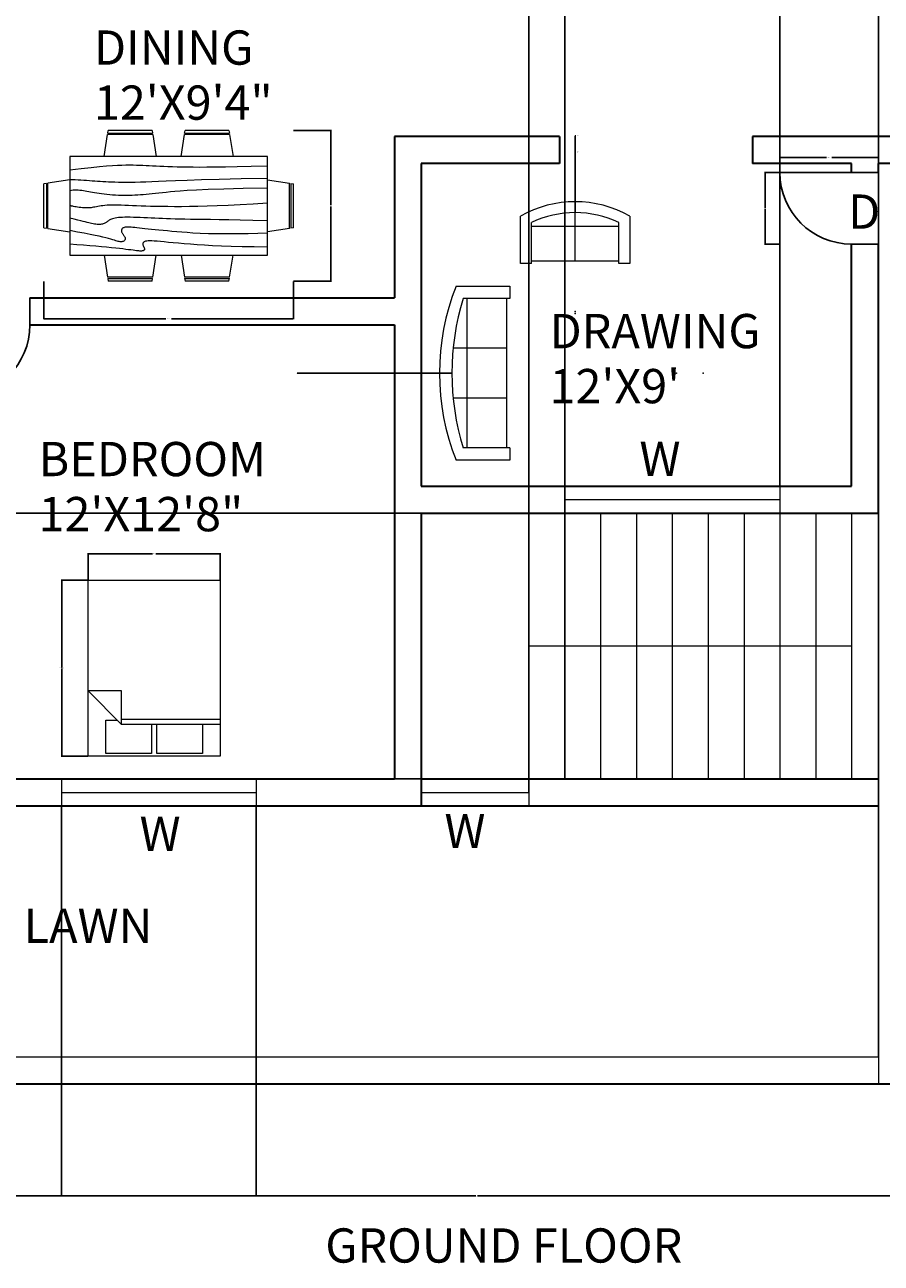
# Model space of a CAD drawing. Units: feet. Extents: x 1889 to 2708, y 1752 to 2375.
# Tile 2 of 5: x 2147 to 2434, y 1752 to 2166. Entities that reach past the tile are written whole.
import ezdxf

# ---------------------------------------------------------------- set-up
doc = ezdxf.new("R2010")
doc.units = ezdxf.units.FT
for name, color, linetype, lineweight in [('A-ANNO-DIMS', 2, 'Continuous', 18), ('A-ANNO-TEXT', 7, 'Continuous', 18), ('A-AREA-IDEN', 7, 'Continuous', 18), ('A-DOOR', 3, 'Continuous', 25), ('A-FLOR-STRS', 7, 'Continuous', 18), ('A-FURN', 8, 'Continuous', 18), ('A-GLAZ', 4, 'Continuous', 18), ('A-WALL', 7, 'Continuous', 35), ('C-PROP', 7, 'Continuous', 30), ('C-SITE', 94, 'Continuous', 18)]:
    doc.layers.add(name, color=color, linetype=linetype, lineweight=lineweight)
doc.styles.get("Standard").update_dxf_attribs({"font": 'arial.ttf'})
doc.dimstyles.get("Standard").update_dxf_attribs({"dimtxt": 0.18, "dimasz": 0.18, "dimexe": 0.18, "dimexo": 0.0625, "dimgap": 0.09, "dimtad": 0, "dimtih": 1, "dimtoh": 1, "dimdec": 4, "dimzin": 0, "dimdsep": 46, "dimtxsty": 'Standard', "dimcen": 0.09, "dimadec": 0, "dimazin": 0, "dimtfac": 1, "dimtdec": 4, "dimtofl": 0, "dimtmove": 0, "dimatfit": 3, "dimfxl": 1, "dimtolj": 1, "dimtzin": 0, "dimarcsym": 0})

# ---------------------------------------------------------------- blocks, each defined once
blk = doc.blocks.new('Dining Set - 36 x 72 in.')
for p, q in [((-22, 27.5), (-22.1562, 26.50042)), ((-22, 27.5), (-6, 27.5)), ((-5.8437, 26.49966), (-6, 27.5)), ((6, 27.5), (5.8438, 26.50042)), ((6, 27.5), (22, 27.5)), ((22.1563, 26.49966), (22, 27.5)), ((-22.2343, 26.00059), (-23.4847, 17.99762)), ((-22.2304, 26), (-5.7608, 26)), ((-5.8416, 26.5), (-22.1534, 26.5)), ((-4.5152, 17.99762), (-5.7655, 25.99926)), ((5.7657, 26.00059), (4.5153, 17.99762)), ((5.7696, 26), (22.2392, 26)), ((22.1584, 26.5), (5.8466, 26.5)), ((23.4848, 17.99762), (22.2345, 25.99926)), ((36, 18), (-36, 18)), ((-36, 18), (-36, -18)), ((36, -18), (36, 18)), ((-44.0006, 8.23428), (-35.9976, 9.48474)), ((44.0006, 8.23428), (35.9976, 9.48474)), ((-45.5, 8), (-44.5004, 8.15617)), ((-45.5, 8), (-45.5, -8)), ((-44.5, -8.15843), (-44.5, 8.15338)), ((-44, 8.23041), (-44, -8.23915)), ((44, 8.23041), (44, -8.23915)), ((44.5, -8.15843), (44.5, 8.15338)), ((45.5, 8), (44.5005, 8.15617)), ((45.5, 8), (45.5, -8)), ((-44.4997, -8.15631), (-45.5, -8)), ((-35.9976, -9.48476), (-43.9993, -8.2345)), ((35.9976, -9.48476), (43.9993, -8.2345)), ((44.4997, -8.15631), (45.5, -8)), ((-36, -18), (36, -18)), ((-22.2343, -26.0006), (-23.4847, -17.99762)), ((-4.5152, -17.99762), (-5.7655, -25.99928)), ((5.7657, -26.0006), (4.5153, -17.99762)), ((23.4848, -17.99762), (22.2345, -25.99928)), ((-22.2304, -26), (-5.7608, -26)), ((-22, -27.5), (-22.1562, -26.50044)), ((-5.8416, -26.5), (-22.1534, -26.5)), ((-5.8437, -26.49967), (-6, -27.5)), ((5.7696, -26), (22.2392, -26)), ((6, -27.5), (5.8438, -26.50044)), ((22.1584, -26.5), (5.8466, -26.5)), ((22.1563, -26.49967), (22, -27.5)), ((-22, -27.5), (-6, -27.5)), ((6, -27.5), (22, -27.5))]:
    blk.add_line(p, q)
for points in [[(-36, 15), (-31.1772, 14.97754), (-26.8079, 14.91406), (-22.8538, 14.81543), (-19.276, 14.6875), (-16.0362, 14.53613), (-13.0957, 14.36718), (-10.4159, 14.18652), (-7.9583, 14), (-5.6904, 13.81315), (-3.6035, 13.63021), (-1.6954, 13.45508), (0.0365, 13.29166), (1.5945, 13.14388), (2.9811, 13.01562), (4.1988, 12.9108), (5.25, 12.83333), (6.1393, 12.78613), (6.8802, 12.76823), (7.4883, 12.77767), (7.9792, 12.8125), (8.3685, 12.87077), (8.6719, 12.95052), (8.9049, 13.0498), (9.0833, 13.16666), (9.2205, 13.29899), (9.3216, 13.44401), (9.3895, 13.59879), (9.4271, 13.76041), (9.4373, 13.92594), (9.4232, 14.09245), (9.3875, 14.257), (9.3333, 14.41666), (9.2638, 14.56917), (9.1836, 14.71484), (9.0975, 14.85465), (9.0104, 14.98958), (8.9272, 15.1206), (8.8529, 15.2487), (8.7922, 15.37483), (8.75, 15.5), (8.7305, 15.62467), (8.7344, 15.74739), (8.7617, 15.86621), (8.8125, 15.97916), (8.8867, 16.08431), (8.9844, 16.17968), (9.1055, 16.26334), (9.25, 16.33333), (9.4189, 16.38802), (9.6172, 16.42708), (9.8506, 16.45052), (10.125, 16.45833), (10.4463, 16.45052), (10.8203, 16.42708), (11.2529, 16.38802), (11.75, 16.33333), (12.3184, 16.26318), (12.9694, 16.17838), (13.7151, 16.07991), (14.5677, 15.96875), (15.5395, 15.84586), (16.6426, 15.71224), (17.8893, 15.56884), (19.2917, 15.41666), (20.859, 15.25667), (22.5879, 15.08984), (24.4721, 14.91715), (26.5052, 14.73958), (28.6809, 14.5581), (30.9929, 14.3737), (33.4347, 14.18733), (36, 14)], [(-36, 10), (-28.9766, 10.14274), (-23.1725, 10.20442), (-18.4241, 10.19775), (-14.5677, 10.13541), (-11.4399, 10.03011), (-8.877, 9.89453), (-6.7154, 9.74137), (-4.7917, 9.58333), (-2.9698, 9.43082), (-1.2246, 9.28515), (0.4415, 9.14534), (2.026, 9.01041), (3.5266, 8.87939), (4.9408, 8.7513), (6.266, 8.62516), (7.5, 8.5), (8.6411, 8.37549), (9.6914, 8.2539), (10.6538, 8.13818), (11.5312, 8.03125), (12.3267, 7.93603), (13.043, 7.85547), (13.6831, 7.79248), (14.25, 7.75), (14.7471, 7.7303), (15.1797, 7.73307), (15.5537, 7.75732), (15.875, 7.80208), (16.1494, 7.86637), (16.3828, 7.94922), (16.5811, 8.04964), (16.75, 8.16666), (16.8944, 8.29915), (17.0143, 8.44531), (17.1089, 8.60319), (17.1771, 8.77083), (17.218, 8.94629), (17.2305, 9.1276), (17.2137, 9.31282), (17.1667, 9.5), (17.0895, 9.6875), (16.987, 9.875), (16.8649, 10.0625), (16.7292, 10.25), (16.5856, 10.4375), (16.4401, 10.625), (16.2985, 10.8125), (16.1667, 11), (16.05, 11.18733), (15.9518, 11.3737), (15.8752, 11.5581), (15.8229, 11.73958), (15.798, 11.91715), (15.8034, 12.08984), (15.842, 12.25667), (15.9167, 12.41666), (16.0295, 12.56836), (16.1784, 12.70833), (16.3605, 12.83268), (16.5729, 12.9375), (16.8127, 13.01888), (17.0768, 13.07291), (17.3625, 13.0957), (17.6667, 13.08333), (17.9894, 13.03312), (18.3418, 12.94726), (18.7382, 12.82918), (19.1927, 12.68229), (19.7195, 12.51001), (20.3327, 12.31575), (21.0465, 12.10294), (21.875, 11.875), (22.8357, 11.63354), (23.959, 11.37304), (25.2786, 11.08618), (26.8282, 10.76562), (28.6414, 10.40405), (30.752, 9.99414), (33.1936, 9.52856), (36, 9)], [(-36, 5.5), (-30.7157, 5.3348), (-26.069, 5.20963), (-21.9946, 5.11767), (-18.4271, 5.05208), (-15.3009, 5.00602), (-12.5508, 4.97265), (-10.1112, 4.94515), (-7.9167, 4.91666), (-5.909, 4.88167), (-4.0586, 4.83984), (-2.3429, 4.79215), (-0.7396, 4.73958), (0.7739, 4.6831), (2.22, 4.6237), (3.6213, 4.56233), (5, 4.5), (6.373, 4.43782), (7.7344, 4.3776), (9.0723, 4.32129), (10.375, 4.27083), (11.6309, 4.22819), (12.8281, 4.19531), (13.9551, 4.17415), (15, 4.16666), (15.954, 4.17448), (16.819, 4.19791), (17.6001, 4.23698), (18.3021, 4.29166), (18.9299, 4.36198), (19.4883, 4.44791), (19.9823, 4.54948), (20.4167, 4.66666), (20.7969, 4.79899), (21.1302, 4.94401), (21.4245, 5.09879), (21.6875, 5.26041), (21.9271, 5.42594), (22.1511, 5.59245), (22.3672, 5.757), (22.5834, 5.91666), (22.8065, 6.06868), (23.0404, 6.21093), (23.2879, 6.34147), (23.5521, 6.45833), (23.8358, 6.55957), (24.142, 6.64323), (24.4735, 6.70735), (24.8334, 6.75), (25.2235, 6.76969), (25.642, 6.76692), (26.0858, 6.74267), (26.5521, 6.69791), (27.0379, 6.63362), (27.5404, 6.55078), (28.0565, 6.45036), (28.5834, 6.33333), (29.1242, 6.19987), (29.7071, 6.04687), (30.3661, 5.87044), (31.1354, 5.66666), (32.0493, 5.43164), (33.142, 5.16146), (34.4475, 4.85221), (36, 4.5)], [(-36, -1), (-30.7915, -0.6591), (-26.0195, -0.38216), (-21.6519, -0.16284), (-17.6563, 0.00521), (-14.0005, 0.12833), (-10.6523, 0.21289), (-7.5796, 0.26522), (-4.75, 0.29166), (-2.134, 0.29793), (0.2878, 0.28711), (2.5317, 0.26163), (4.6146, 0.22396), (6.5529, 0.17651), (8.3633, 0.12174), (10.0623, 0.06209), (11.6667, 0), (13.1899, -0.06201), (14.6341, -0.1211), (15.9982, -0.17432), (17.2813, -0.21875), (18.4823, -0.25147), (19.6003, -0.26953), (20.6343, -0.27002), (21.5834, -0.25), (22.4481, -0.20768), (23.2357, -0.14584), (23.9549, -0.06836), (24.6146, 0.02083), (25.2235, 0.11784), (25.7904, 0.21875), (26.3241, 0.31966), (26.8334, 0.41666), (27.3265, 0.50618), (27.8099, 0.58593), (28.2894, 0.65397), (28.7709, 0.70833), (29.2601, 0.74707), (29.763, 0.76823), (30.2855, 0.76985), (30.8334, 0.75), (31.4088, 0.70784), (31.9994, 0.64713), (32.589, 0.57275), (33.1615, 0.48958), (33.7008, 0.4025), (34.1908, 0.3164), (34.6153, 0.23616), (34.9584, 0.16666), (35.2099, 0.11165), (35.3848, 0.07031), (35.504, 0.04069), (35.5886, 0.02083), (35.6594, 0.00879), (35.7377, 0.0026), (35.8442, 0.00032), (36, 0)], [(-36, -6.5), (-27.1843, -6.31267), (-20.084, -6.1263), (-14.469, -5.9419), (-10.1094, -5.76042), (-6.7752, -5.58285), (-4.2363, -5.41016), (-2.2629, -5.24333), (-0.625, -5.08334), (0.8708, -4.93099), (2.2715, -4.78646), (3.5872, -4.64974), (4.8281, -4.52084), (6.0046, -4.39974), (7.127, -4.28646), (8.2053, -4.18099), (9.25, -4.08334), (10.2705, -3.99382), (11.2734, -3.91407), (12.2647, -3.84603), (13.25, -3.79167), (14.2354, -3.75293), (15.2266, -3.73177), (16.2295, -3.73015), (17.25, -3.75), (18.2912, -3.79248), (19.3451, -3.85547), (20.4009, -3.93604), (21.4479, -4.03125), (22.4754, -4.13819), (23.4727, -4.25391), (24.4289, -4.37549), (25.3334, -4.5), (26.1785, -4.62492), (26.9694, -4.74935), (27.7145, -4.87281), (28.4219, -4.99479), (29.1, -5.11483), (29.7572, -5.23242), (30.4016, -5.34709), (31.0417, -5.45834), (31.6837, -5.56437), (32.3262, -5.65821), (32.9658, -5.73153), (33.599, -5.77604), (34.2224, -5.78345), (34.8327, -5.74545), (35.4264, -5.65373), (36, -5.5)], [(-36, -10), (-26.4022, -9.81299), (-18.4675, -9.62891), (-11.9839, -9.45069), (-6.7396, -9.28125), (-2.5226, -9.12354), (0.8789, -8.98047), (3.6769, -8.85498), (6.0833, -8.75), (8.2767, -8.66765), (10.3021, -8.60677), (12.1712, -8.56543), (13.8958, -8.54167), (15.4876, -8.53353), (16.9583, -8.53907), (18.3197, -8.55632), (19.5834, -8.58334), (20.7616, -8.61841), (21.8685, -8.66081), (22.9188, -8.71004), (23.9271, -8.76563), (24.9081, -8.82707), (25.8763, -8.89388), (26.8465, -8.96558), (27.8334, -9.04167), (28.8474, -9.12118), (29.8828, -9.20117), (30.93, -9.27824), (31.9792, -9.34896), (33.0205, -9.40991), (34.0443, -9.45768), (35.0407, -9.48885), (36, -9.5)], [(-36, -14.5), (-30.0881, -14.33513), (-25.0332, -14.21224), (-20.7312, -14.12647), (-17.0781, -14.07292), (-13.97, -14.04671), (-11.3027, -14.04297), (-8.9724, -14.05681), (-6.875, -14.08334), (-4.9224, -14.11833), (-3.0905, -14.16016), (-1.3709, -14.20785), (0.2448, -14.26042), (1.7647, -14.3169), (3.1973, -14.3763), (4.5507, -14.43767), (5.8333, -14.5), (7.0554, -14.5621), (8.235, -14.62175), (9.3922, -14.67652), (10.5469, -14.72396), (11.7192, -14.76164), (12.929, -14.78711), (14.1965, -14.79794), (15.5417, -14.79167), (16.9933, -14.76424), (18.6152, -14.70508), (20.4804, -14.60197), (22.6615, -14.44271), (25.2312, -14.21509), (28.2624, -13.9069), (31.8277, -13.50594), (36, -13)]]:
    blk.add_lwpolyline(points)
blk = doc.blocks.new('Bed - Queen')
for p, q in [((0, -80.00003), (0, 0)), ((0, 0), (59.99999, 0)), ((59.99999, 0), (59.99999, -80.00003)), ((7.99999, -1.2), (28.79998, -1.2)), ((7.99999, -14.4), (7.99999, -1.2)), ((28.79998, -1.2), (28.79998, -14.4)), ((31.19999, -1.2), (51.99999, -1.2)), ((31.19999, -14.4), (31.19999, -1.2)), ((51.99999, -1.2), (51.99999, -16.4)), ((0, -14.4), (44.8, -14.4)), ((44.8, -16.8), (0, -16.8)), ((59.99999, -29.6), (44.8, -14.4)), ((44.8, -14.4), (44.8, -29.6)), ((51.99999, -16.4), (46.79936, -16.4)), ((44.8, -29.6), (59.99999, -29.6)), ((59.99999, -80.00003), (0, -80.00003))]:
    blk.add_line(p, q)
blk = doc.blocks.new('Sofa - Roundback 7 ft.')
for p, q in [((-36.000027, -34), (-36.000027, -11.4696)), ((-12.00002, -32.4421), (-12.00003, -6.5971)), ((11.99997, -32.4421), (11.99998, -6.5971)), ((35.99998, -34), (35.99998, -11.4696)), ((-35.999844, -13.3819), (35.9998, -13.3819)), ((-36.000027, -32.4421), (35.99998, -32.4421))]:
    blk.add_line(p, q)
for points in [[(-36.000027, -34), (-42.000027, -34), (-42.000027, -8)], [(41.99998, -8), (41.99998, -34), (35.99998, -34)]]:
    blk.add_lwpolyline(points)
for centre, radius, start, end in [((0, -114.25), 114.25, 68.43141, 111.5686), ((-0.00001, -127.1968), 121.1968, 72.72033, 107.2797)]:
    blk.add_arc(centre, radius, start, end)
blk = doc.blocks.new('Sofa - Roundback Loveseat 5 ft.')
for p, q in [((0, -32.44198), (0, -5.99998)), ((-24, -33.99998), (-24, -11.46958)), ((-23.9998, -13.38178), (23.99986, -13.38178)), ((24.00004, -33.99998), (24.00004, -11.46958)), ((-24, -32.44198), (24.00004, -32.44198))]:
    blk.add_line(p, q)
for points in [[(-24, -33.99998), (-30, -33.99998), (-30, -7.99998)], [(30.00004, -7.99998), (30.00004, -33.99998), (24.00004, -33.99998)]]:
    blk.add_lwpolyline(points)
for centre, radius, start, end in [((0, -60.24998), 60.24998, 60.13715, 119.8628), ((0, -61.38438), 55.38444, 64.32083, 115.6792)]:
    blk.add_arc(centre, radius, start, end)
blk = doc.blocks.new('DOOR-SWING-24')
for p, q in [((9, 24), (0, 24)), ((33, 0), (0, 0))]:
    blk.add_line(p, q)
blk.add_arc((9, 0), 24, 0, 90)
blk = doc.blocks.new('*D13')
at = {"layer": 'A-ANNO-DIMS', "color": 0, "lineweight": -2, "transparency": 16777216}
for p, q in [((2399.86, 2116.66), (2399.86, 2121.73)), ((2400.04, 2121.55), (2415.43, 2121.55)), ((2432.68, 2121.55), (2417.3, 2121.55)), ((2432.86, 2116.66), (2432.86, 2121.73))]:
    blk.add_line(p, q, dxfattribs=at)
at = {"layer": 'A-ANNO-DIMS', "color": 0, "transparency": 16777216}
for points in [[(2400.04, 2121.58), (2400.04, 2121.52), (2399.86, 2121.55)], [(2432.68, 2121.58), (2432.68, 2121.52), (2432.86, 2121.55)]]:
    blk.add_solid(points, dxfattribs=at)
at = {"layer": 'Defpoints', "color": 0, "transparency": 16777216}
for p in [(2399.86, 2121.55), (2399.86, 2116.6), (2432.86, 2116.6)]:
    blk.add_point(p, dxfattribs=at)
at = {"layer": 'A-ANNO-DIMS', "color": 0, "transparency": 16777216, "insert": (2416.36, 2121.55), "char_height": 0.18, "attachment_point": 5}
blk.add_mtext('\\A1;DOOR 33 TYP.', dxfattribs=at)
blk = doc.blocks.new('*D14')
at = {"layer": 'A-ANNO-DIMS', "color": 0, "lineweight": -2, "transparency": 16777216}
for p, q in [((2399.8, 2116.6), (2394.73, 2116.6)), ((2394.91, 2116.42), (2394.91, 2104.78)), ((2394.91, 2092.78), (2394.91, 2104.42)), ((2399.8, 2092.6), (2394.73, 2092.6))]:
    blk.add_line(p, q, dxfattribs=at)
at = {"layer": 'A-ANNO-DIMS', "color": 0, "transparency": 16777216}
for points in [[(2394.88, 2116.42), (2394.94, 2116.42), (2394.91, 2116.6)], [(2394.88, 2092.78), (2394.94, 2092.78), (2394.91, 2092.6)]]:
    blk.add_solid(points, dxfattribs=at)
at = {"layer": 'Defpoints', "color": 0, "transparency": 16777216}
for p in [(2399.86, 2116.6), (2394.91, 2092.6), (2399.86, 2092.6)]:
    blk.add_point(p, dxfattribs=at)
at = {"layer": 'A-ANNO-DIMS', "color": 0, "transparency": 16777216, "insert": (2394.91, 2104.6), "char_height": 0.18, "attachment_point": 5}
blk.add_mtext('\\A1;24 TYP.', dxfattribs=at)
blk = doc.blocks.new('*D19')
at = {"layer": 'A-ANNO-DIMS', "color": 0, "lineweight": -2, "transparency": 16777216}
for p, q in [((2168.27, 1980.15), (2159.31, 1980.15)), ((2159.49, 1979.97), (2159.49, 1950.88)), ((2159.49, 1921.43), (2159.49, 1950.52)), ((2168.27, 1921.25), (2159.31, 1921.25))]:
    blk.add_line(p, q, dxfattribs=at)
at = {"layer": 'A-ANNO-DIMS', "color": 0, "transparency": 16777216}
for points in [[(2159.46, 1979.97), (2159.52, 1979.97), (2159.49, 1980.15)], [(2159.46, 1921.43), (2159.52, 1921.43), (2159.49, 1921.25)]]:
    blk.add_solid(points, dxfattribs=at)
at = {"layer": 'Defpoints', "color": 0, "transparency": 16777216}
for p in [(2168.33, 1980.15), (2159.49, 1921.25), (2168.33, 1921.25)]:
    blk.add_point(p, dxfattribs=at)
at = {"layer": 'A-ANNO-DIMS', "color": 0, "transparency": 16777216, "insert": (2159.49, 1950.7), "char_height": 0.18, "attachment_point": 5}
blk.add_mtext('\\A1;BED 59 TYP.', dxfattribs=at)
blk = doc.blocks.new('*D20')
at = {"layer": 'A-ANNO-DIMS', "color": 0, "lineweight": -2, "transparency": 16777216}
for p, q in [((2168.33, 1980.22), (2168.33, 1989.17)), ((2168.51, 1988.99), (2189.89, 1988.99)), ((2212.33, 1988.99), (2190.95, 1988.99)), ((2212.51, 1980.22), (2212.51, 1989.17))]:
    blk.add_line(p, q, dxfattribs=at)
at = {"layer": 'A-ANNO-DIMS', "color": 0, "transparency": 16777216}
for points in [[(2168.51, 1989.02), (2168.51, 1988.96), (2168.33, 1988.99)], [(2212.33, 1989.02), (2212.33, 1988.96), (2212.51, 1988.99)]]:
    blk.add_solid(points, dxfattribs=at)
at = {"layer": 'Defpoints', "color": 0, "transparency": 16777216}
for p in [(2168.33, 1988.99), (2168.33, 1980.15), (2212.51, 1980.15)]:
    blk.add_point(p, dxfattribs=at)
at = {"layer": 'A-ANNO-DIMS', "color": 0, "transparency": 16777216, "insert": (2190.42, 1988.99), "char_height": 0.18, "attachment_point": 5}
blk.add_mtext('\\A1;44 TYP.', dxfattribs=at)
blk = doc.blocks.new('*D31')
at = {"layer": 'A-ANNO-DIMS', "color": 0, "lineweight": -2, "transparency": 16777216}
for p, q in [((2153.5, 2080.07), (2153.5, 2067.42)), ((2237.06, 2080.07), (2237.06, 2067.42)), ((2153.68, 2067.6), (2194.31, 2067.6)), ((2236.88, 2067.6), (2196.25, 2067.6))]:
    blk.add_line(p, q, dxfattribs=at)
at = {"layer": 'A-ANNO-DIMS', "color": 0, "transparency": 16777216}
for points in [[(2153.68, 2067.63), (2153.68, 2067.57), (2153.5, 2067.6)], [(2236.88, 2067.63), (2236.88, 2067.57), (2237.06, 2067.6)]]:
    blk.add_solid(points, dxfattribs=at)
at = {"layer": 'Defpoints', "color": 0, "transparency": 16777216}
for p in [(2153.5, 2080.14), (2237.06, 2080.14), (2153.5, 2067.6)]:
    blk.add_point(p, dxfattribs=at)
at = {"layer": 'A-ANNO-DIMS', "color": 0, "transparency": 16777216, "insert": (2195.28, 2067.6), "char_height": 0.18, "attachment_point": 5}
blk.add_mtext('\\A1;DINING SET 84', dxfattribs=at)
blk = doc.blocks.new('*D32')
at = {"layer": 'A-ANNO-DIMS', "color": 0, "lineweight": -2, "transparency": 16777216}
for p, q in [((2237.13, 2130.64), (2249.78, 2130.64)), ((2249.6, 2130.46), (2249.6, 2105.57)), ((2249.6, 2080.32), (2249.6, 2105.21)), ((2237.13, 2080.14), (2249.78, 2080.14))]:
    blk.add_line(p, q, dxfattribs=at)
at = {"layer": 'A-ANNO-DIMS', "color": 0, "transparency": 16777216}
for points in [[(2249.57, 2130.46), (2249.63, 2130.46), (2249.6, 2130.64)], [(2249.57, 2080.32), (2249.63, 2080.32), (2249.6, 2080.14)]]:
    blk.add_solid(points, dxfattribs=at)
at = {"layer": 'Defpoints', "color": 0, "transparency": 16777216}
for p in [(2237.06, 2130.64), (2237.06, 2080.14), (2249.6, 2080.14)]:
    blk.add_point(p, dxfattribs=at)
at = {"layer": 'A-ANNO-DIMS', "color": 0, "transparency": 16777216, "insert": (2249.6, 2105.39), "char_height": 0.18, "attachment_point": 5}
blk.add_mtext('\\A1;51', dxfattribs=at)
blk = doc.blocks.new('*D44')
at = {"layer": 'A-ANNO-DIMS', "color": 0, "lineweight": -2, "transparency": 16777216}
for p, q in [((1926.86, 1811.54), (1926.86, 1773.87)), ((2669.86, 1811.54), (2669.86, 1773.87)), ((1927.04, 1774.05), (2298.08, 1774.05)), ((2669.68, 1774.05), (2298.65, 1774.05))]:
    blk.add_line(p, q, dxfattribs=at)
at = {"layer": 'A-ANNO-DIMS', "color": 0, "transparency": 16777216}
for points in [[(1927.04, 1774.08), (1927.04, 1774.02), (1926.86, 1774.05)], [(2669.68, 1774.08), (2669.68, 1774.02), (2669.86, 1774.05)]]:
    blk.add_solid(points, dxfattribs=at)
at = {"layer": 'Defpoints', "color": 0, "transparency": 16777216}
for p in [(1926.86, 1811.6), (2669.86, 1811.6), (2669.86, 1774.05)]:
    blk.add_point(p, dxfattribs=at)
at = {"layer": 'A-ANNO-DIMS', "color": 0, "transparency": 16777216, "insert": (2298.36, 1774.05), "char_height": 0.18, "attachment_point": 5}
blk.add_mtext('\\A1;743', dxfattribs=at)
blk = doc.blocks.new('*D48')
at = {"layer": 'A-ANNO-DIMS', "color": 0, "lineweight": -2, "transparency": 16777216}
for p, q in [((1983.86, 1820.66), (1983.86, 2375.33)), ((1984.04, 2375.15), (2208.07, 2375.15)), ((2432.68, 2375.15), (2208.66, 2375.15)), ((2432.86, 1820.66), (2432.86, 2375.33))]:
    blk.add_line(p, q, dxfattribs=at)
at = {"layer": 'A-ANNO-DIMS', "color": 0, "transparency": 16777216}
for points in [[(1984.04, 2375.18), (1984.04, 2375.12), (1983.86, 2375.15)], [(2432.68, 2375.18), (2432.68, 2375.12), (2432.86, 2375.15)]]:
    blk.add_solid(points, dxfattribs=at)
at = {"layer": 'Defpoints', "color": 0, "transparency": 16777216}
for p in [(2432.86, 2375.15), (1983.86, 1820.6), (2432.86, 1820.6)]:
    blk.add_point(p, dxfattribs=at)
at = {"layer": 'A-ANNO-DIMS', "color": 0, "transparency": 16777216, "insert": (2208.36, 2375.15), "char_height": 0.18, "attachment_point": 5}
blk.add_mtext('\\A1;449', dxfattribs=at)
blk = doc.blocks.new('*D58')
at = {"layer": 'A-ANNO-DIMS', "color": 0, "lineweight": -2, "transparency": 16777216}
for p, q in [((1983.86, 1904.54), (1983.86, 1773.87)), ((2159.47, 1904.54), (2159.47, 1773.87)), ((1984.04, 1774.05), (2071.28, 1774.05)), ((2159.29, 1774.05), (2072.05, 1774.05))]:
    blk.add_line(p, q, dxfattribs=at)
at = {"layer": 'A-ANNO-DIMS', "color": 0, "transparency": 16777216}
for points in [[(1984.04, 1774.08), (1984.04, 1774.02), (1983.86, 1774.05)], [(2159.29, 1774.08), (2159.29, 1774.02), (2159.47, 1774.05)]]:
    blk.add_solid(points, dxfattribs=at)
at = {"layer": 'Defpoints', "color": 0, "transparency": 16777216}
for p in [(1983.86, 1904.6), (2159.47, 1904.6), (2159.47, 1774.05)]:
    blk.add_point(p, dxfattribs=at)
at = {"layer": 'A-ANNO-DIMS', "color": 0, "transparency": 16777216, "insert": (2071.67, 1774.05), "char_height": 0.18, "attachment_point": 5}
blk.add_mtext('\\A1;175.6', dxfattribs=at)
blk = doc.blocks.new('*D59')
at = {"layer": 'A-ANNO-DIMS', "color": 0, "lineweight": -2, "transparency": 16777216}
for p, q in [((2159.47, 1904.54), (2159.47, 1773.87)), ((2224.63, 1904.54), (2224.63, 1773.87)), ((2159.65, 1774.05), (2191.65, 1774.05)), ((2224.45, 1774.05), (2192.44, 1774.05))]:
    blk.add_line(p, q, dxfattribs=at)
at = {"layer": 'A-ANNO-DIMS', "color": 0, "transparency": 16777216}
for points in [[(2159.65, 1774.08), (2159.65, 1774.02), (2159.47, 1774.05)], [(2224.45, 1774.08), (2224.45, 1774.02), (2224.63, 1774.05)]]:
    blk.add_solid(points, dxfattribs=at)
at = {"layer": 'Defpoints', "color": 0, "transparency": 16777216}
for p in [(2159.47, 1904.6), (2224.63, 1904.6), (2224.63, 1774.05)]:
    blk.add_point(p, dxfattribs=at)
at = {"layer": 'A-ANNO-DIMS', "color": 0, "transparency": 16777216, "insert": (2192.05, 1774.05), "char_height": 0.18, "attachment_point": 5}
blk.add_mtext('\\A1;65.16', dxfattribs=at)
blk = doc.blocks.new('*D60')
at = {"layer": 'A-ANNO-DIMS', "color": 0, "lineweight": -2, "transparency": 16777216}
for p, q in [((2423.8, 2002.6), (1889.13, 2002.6)), ((1889.31, 2002.42), (1889.31, 1958.28)), ((1889.31, 1913.78), (1889.31, 1957.92)), ((2423.8, 1913.6), (1889.13, 1913.6))]:
    blk.add_line(p, q, dxfattribs=at)
at = {"layer": 'A-ANNO-DIMS', "color": 0, "transparency": 16777216}
for points in [[(1889.28, 2002.42), (1889.34, 2002.42), (1889.31, 2002.6)], [(1889.28, 1913.78), (1889.34, 1913.78), (1889.31, 1913.6)]]:
    blk.add_solid(points, dxfattribs=at)
at = {"layer": 'Defpoints', "color": 0, "transparency": 16777216}
for p in [(1889.31, 2002.6), (2423.86, 2002.6), (2423.86, 1913.6)]:
    blk.add_point(p, dxfattribs=at)
at = {"layer": 'A-ANNO-DIMS', "color": 0, "transparency": 16777216, "insert": (1889.31, 1958.1), "char_height": 0.18, "attachment_point": 5}
blk.add_mtext('\\A1;89', dxfattribs=at)
blk = doc.blocks.new('*D61')
at = {"layer": 'A-ANNO-DIMS', "color": 0, "lineweight": -2, "transparency": 16777216}
for p, q in [((2315.86, 1909.16), (2315.86, 2375.33)), ((2316.04, 2375.15), (2321.65, 2375.15)), ((2327.68, 2375.15), (2322.07, 2375.15)), ((2327.86, 1913.66), (2327.86, 2375.33))]:
    blk.add_line(p, q, dxfattribs=at)
at = {"layer": 'A-ANNO-DIMS', "color": 0, "transparency": 16777216}
for points in [[(2316.04, 2375.18), (2316.04, 2375.12), (2315.86, 2375.15)], [(2327.68, 2375.18), (2327.68, 2375.12), (2327.86, 2375.15)]]:
    blk.add_solid(points, dxfattribs=at)
at = {"layer": 'Defpoints', "color": 0, "transparency": 16777216}
for p in [(2327.86, 2375.15), (2327.86, 1913.6), (2315.86, 1909.1)]:
    blk.add_point(p, dxfattribs=at)
at = {"layer": 'A-ANNO-DIMS', "color": 0, "transparency": 16777216, "insert": (2321.86, 2375.15), "char_height": 0.18, "attachment_point": 5}
blk.add_mtext('\\A1;12', dxfattribs=at)
blk = doc.blocks.new('*D64')
at = {"layer": 'A-ANNO-DIMS', "color": 0, "lineweight": -2, "transparency": 16777216}
for p, q in [((2327.86, 2011.66), (2327.86, 2375.33)), ((2328.04, 2375.15), (2363.65, 2375.15)), ((2399.68, 2375.15), (2364.08, 2375.15)), ((2399.86, 2011.66), (2399.86, 2375.33))]:
    blk.add_line(p, q, dxfattribs=at)
at = {"layer": 'A-ANNO-DIMS', "color": 0, "transparency": 16777216}
for points in [[(2328.04, 2375.18), (2328.04, 2375.12), (2327.86, 2375.15)], [(2399.68, 2375.18), (2399.68, 2375.12), (2399.86, 2375.15)]]:
    blk.add_solid(points, dxfattribs=at)
at = {"layer": 'Defpoints', "color": 0, "transparency": 16777216}
for p in [(2399.86, 2375.15), (2327.86, 2011.6), (2399.86, 2011.6)]:
    blk.add_point(p, dxfattribs=at)
at = {"layer": 'A-ANNO-DIMS', "color": 0, "transparency": 16777216, "insert": (2363.86, 2375.15), "char_height": 0.18, "attachment_point": 5}
blk.add_mtext('\\A1;72', dxfattribs=at)
blk = doc.blocks.new('*D67')
at = {"layer": 'A-ANNO-DIMS', "color": 0, "lineweight": -2, "transparency": 16777216}
for p, q in [((2239.61, 2049.39), (2289.9, 2049.39)), ((2374.12, 2049.39), (2374.3, 2049.39)), ((2374.21, 2049.3), (2374.21, 2049.48))]:
    blk.add_line(p, q, dxfattribs=at)
at = {"layer": 'A-ANNO-DIMS', "color": 0, "transparency": 16777216}
blk.add_solid([(2289.9, 2049.42), (2289.9, 2049.36), (2290.08, 2049.39)], dxfattribs=at)
at = {"layer": 'Defpoints', "color": 0, "transparency": 16777216}
for p in [(2290.08, 2049.39), (2374.21, 2049.39)]:
    blk.add_point(p, dxfattribs=at)
at = {"layer": 'A-ANNO-DIMS', "color": 0, "transparency": 16777216, "insert": (2238.94, 2049.39), "char_height": 0.18, "attachment_point": 5}
blk.add_mtext('\\A1;2X R84.12', dxfattribs=at)
blk = doc.blocks.new('*D68')
at = {"layer": 'A-ANNO-DIMS', "color": 0, "lineweight": -2, "transparency": 16777216}
for p, q in [((2238.34, 2049.39), (2285.74, 2049.39)), ((2365.13, 2049.39), (2365.31, 2049.39)), ((2365.22, 2049.3), (2365.22, 2049.48))]:
    blk.add_line(p, q, dxfattribs=at)
at = {"layer": 'A-ANNO-DIMS', "color": 0, "transparency": 16777216}
blk.add_solid([(2285.74, 2049.42), (2285.74, 2049.36), (2285.92, 2049.39)], dxfattribs=at)
at = {"layer": 'Defpoints', "color": 0, "transparency": 16777216}
for p in [(2285.92, 2049.39), (2365.22, 2049.39)]:
    blk.add_point(p, dxfattribs=at)
at = {"layer": 'A-ANNO-DIMS', "color": 0, "transparency": 16777216, "insert": (2237.73, 2049.39), "char_height": 0.18, "attachment_point": 5}
blk.add_mtext('\\A1;2X R79.3', dxfattribs=at)
blk = doc.blocks.new('*D69')
at = {"layer": 'A-ANNO-DIMS', "color": 0, "lineweight": -2, "transparency": 16777216}
for p, q in [((2331.53, 2128.85), (2331.35, 2128.85)), ((2331.35, 2128.85), (2331.34, 2106.98)), ((2331.25, 2070.04), (2331.43, 2070.04)), ((2331.34, 2069.95), (2331.34, 2070.13))]:
    blk.add_line(p, q, dxfattribs=at)
at = {"layer": 'A-ANNO-DIMS', "color": 0, "transparency": 16777216}
blk.add_solid([(2331.32, 2106.98), (2331.38, 2106.98), (2331.34, 2106.8)], dxfattribs=at)
at = {"layer": 'Defpoints', "color": 0, "transparency": 16777216}
for p in [(2331.34, 2106.8), (2331.34, 2070.04)]:
    blk.add_point(p, dxfattribs=at)
at = {"layer": 'A-ANNO-DIMS', "color": 0, "transparency": 16777216, "insert": (2332.27, 2128.85), "char_height": 0.18, "attachment_point": 5}
blk.add_mtext('\\A1;2X R36.755', dxfattribs=at)
blk = doc.blocks.new('*D70')
at = {"layer": 'A-ANNO-DIMS', "color": 0, "lineweight": -2, "transparency": 16777216}
for p, q in [((2331.53, 2123.41), (2331.35, 2123.41)), ((2331.35, 2123.41), (2331.34, 2103.32)), ((2331.25, 2069.35), (2331.43, 2069.35)), ((2331.34, 2069.26), (2331.34, 2069.44))]:
    blk.add_line(p, q, dxfattribs=at)
at = {"layer": 'A-ANNO-DIMS', "color": 0, "transparency": 16777216}
blk.add_solid([(2331.32, 2103.32), (2331.38, 2103.32), (2331.34, 2103.14)], dxfattribs=at)
at = {"layer": 'Defpoints', "color": 0, "transparency": 16777216}
for p in [(2331.34, 2103.14), (2331.34, 2069.35)]:
    blk.add_point(p, dxfattribs=at)
at = {"layer": 'A-ANNO-DIMS', "color": 0, "transparency": 16777216, "insert": (2332.2, 2123.41), "char_height": 0.18, "attachment_point": 5}
blk.add_mtext('\\A1;2X R33.79', dxfattribs=at)

msp = doc.modelspace()

# ---------------------------------------------------------------- linework, layer by layer
at = {"layer": 'A-FLOR-STRS'}
for p, q in [((2327.8644, 2011.5988), (2327.8644, 1913.5988)), ((2399.8644, 2011.5988), (2399.8644, 1913.5988)), ((2315.8644, 2002.5988), (2315.8644, 1904.5988)), ((2339.8644, 2002.5988), (2339.8644, 1913.5988)), ((2351.8644, 2002.5988), (2351.8644, 1913.5988)), ((2363.8644, 2002.5988), (2363.8644, 1913.5988)), ((2375.8644, 2002.5988), (2375.8644, 1913.5988)), ((2387.8644, 2002.5988), (2387.8644, 1913.5988)), ((2411.8644, 2002.5988), (2411.8644, 1913.5988)), ((2423.8644, 2002.5988), (2423.8644, 1913.5988)), ((2315.8644, 1958.0988), (2423.8644, 1958.0988))]:
    msp.add_line(p, q, dxfattribs=at)
at = {"layer": 'A-GLAZ'}
for p, q in [((2327.8644, 2007.0988), (2399.8644, 2007.0988)), ((2159.4686, 1913.5988), (2159.4686, 1904.5988)), ((2224.6291, 1913.5988), (2224.6291, 1904.5988)), ((2159.4686, 1909.0988), (2224.6291, 1909.0988)), ((2279.8644, 1909.0988), (2315.8644, 1909.0988))]:
    msp.add_line(p, q, dxfattribs=at)
at = {"layer": 'A-WALL'}
for p, q in [((2270.8644, 2128.5988), (2270.8644, 2074.5988)), ((2326.1633, 2128.5988), (2270.8644, 2128.5988)), ((2326.1633, 2128.5988), (2326.1633, 2119.5988)), ((2452.8644, 2128.5988), (2390.7022, 2128.5988)), ((2390.7022, 2128.5988), (2390.7022, 2119.5988)), ((2279.8644, 2119.5988), (2279.8644, 2011.5988)), ((2279.8644, 2119.5988), (2279.8644, 2011.5988)), ((2326.1633, 2119.5988), (2279.8644, 2119.5988)), ((2423.8644, 2119.5988), (2390.7022, 2119.5988)), ((2423.8644, 2116.5988), (2423.8644, 2119.5988)), ((2452.8644, 2119.5988), (2432.8644, 2119.5988)), ((2452.8644, 2119.5988), (2432.8644, 2119.5988)), ((2432.8644, 2116.5988), (2432.8644, 2119.5988)), ((2423.8644, 2011.5988), (2423.8644, 2092.5988)), ((2432.8644, 2002.5988), (2432.8644, 2092.5988)), ((2148.8644, 2074.5988), (2270.8644, 2074.5988)), ((2148.8644, 2065.5988), (2270.8644, 2065.5988)), ((2270.8644, 2065.5988), (2270.8644, 1913.5988)), ((2279.8644, 2011.5988), (2423.8644, 2011.5988)), ((2279.8644, 2002.5988), (2432.8644, 2002.5988)), ((2279.8644, 2002.5988), (2279.8644, 1904.5988)), ((2121.8644, 1913.5988), (2270.8644, 1913.5988)), ((2279.8644, 1913.5988), (2432.8644, 1913.5988)), ((2121.8644, 1904.5988), (2432.8644, 1904.5988))]:
    msp.add_line(p, q, dxfattribs=at)
at = {"layer": 'C-PROP'}
for p, q in [((1983.8644, 1811.5988), (2432.8644, 1811.5988)), ((2432.8644, 1811.5988), (2669.8644, 1811.5988))]:
    msp.add_line(p, q, dxfattribs=at)
at = {"layer": 'C-SITE'}
for p, q in [((2432.8644, 1913.5988), (2432.8644, 1811.5988)), ((1983.8644, 1820.5988), (2432.8644, 1820.5988))]:
    msp.add_line(p, q, dxfattribs=at)

# ---------------------------------------------------------------- block references
at = {"layer": 'A-DOOR'}
for p, rotation in [((2432.8649, 2116.5986), 180), ((2124.8647, 2074.5992), 269.9999999999978)]:
    msp.add_blockref('DOOR-SWING-24', p, dxfattribs=dict(at, rotation=rotation))
at = {"layer": 'A-FURN'}
for name, p, xscale, yscale, zscale, rotation in [('Dining Set - 36 x 72 in.', (2195.2807, 2105.3889), 0.918293308787666, 0.918293308787666, 0.918293308787666, 180), ('Sofa - Roundback 7 ft.', (2285.92, 2049.3907), 0.694114071376089, 0.694114071376089, 0.694114071376089, 90), ('Bed - Queen', (2212.5091, 1921.2477), 0.7363101783767424, 0.7363101783767424, 0.7363101783767424, 180)]:
    msp.add_blockref(name, p, dxfattribs=dict(at, xscale=xscale, yscale=yscale, zscale=zscale, rotation=rotation))
at = {"layer": 'A-FURN', "xscale": 0.6100416467231381, "yscale": 0.6100416467231381, "zscale": 0.6100416467231381}
msp.add_blockref('Sofa - Roundback Loveseat 5 ft.', (2331.3448, 2106.7959), dxfattribs=at)

# ---------------------------------------------------------------- texts
at = {"layer": 'A-ANNO-TEXT'}
for s, height, p in [('D', 11.4692, (2422.7158, 2097.7293)), ('W', 11.4692, (2352.8731, 2014.9665)), ('W', 11.4692, (2185.5558, 1889.5243)), ('W', 11.4692, (2287.5993, 1890.4554)), ('GROUND FLOOR', 11.469207, (2247.7163, 1751.7354))]:
    msp.add_text(s, height=height, dxfattribs=at).set_placement(p)
at = {"layer": 'A-AREA-IDEN'}
for s, p in [('DINING', (2170.2832, 2152.6328)), ('12\'X9\'4"', (2170.2832, 2134.2086)), ('DRAWING', (2322.7815, 2057.7543)), ("12'X9'", (2322.7815, 2039.3301)), ('BEDROOM', (2151.746, 2014.9212)), ('12\'X12\'8"', (2151.746, 1996.4969)), ('LAWN', (2146.7975, 1858.7551))]:
    msp.add_text(s, height=11.46921, dxfattribs=at).set_placement(p)

# ---------------------------------------------------------------- dimensions: what is measured, and where the dimension line sits
at = {"layer": 'A-ANNO-DIMS'}
for base, p1, p2, override, picture, middle in [((2432.8644, 2375.1488), (1983.8644, 1820.5988), (2432.8644, 1820.5988), {"dimdec": 0, "dimlfac": 1, "dimrnd": 0, "dimzin": 0, "dimdsep": 46, "dimlunit": 2}, '*D48', (2208.3644, 2375.1488)), ((2327.8644, 2375.1488), (2315.8644, 1909.0988), (2327.8644, 1913.5988), {"dimdec": 0, "dimlfac": 1, "dimrnd": 0, "dimzin": 0, "dimdsep": 46, "dimlunit": 2}, '*D61', (2321.8644, 2375.1488)), ((2399.8644, 2375.1488), (2327.8644, 2011.5988), (2399.8644, 2011.5988), {"dimdec": 0, "dimlfac": 1, "dimrnd": 0, "dimzin": 0, "dimdsep": 46, "dimlunit": 2}, '*D64', (2363.8644, 2375.1488)), ((2159.4686, 1774.0488), (1983.8644, 1904.5988), (2159.4686, 1904.5988), {"dimdec": 1, "dimlfac": 1, "dimrnd": 0, "dimzin": 0, "dimdsep": 46, "dimlunit": 2}, '*D58', (2071.6665, 1774.0488)), ((2224.6291, 1774.0488), (2159.4686, 1904.5988), (2224.6291, 1904.5988), {"dimdec": 2, "dimlfac": 1, "dimrnd": 0, "dimzin": 0, "dimdsep": 46, "dimlunit": 2}, '*D59', (2192.0488, 1774.0488)), ((2669.8644, 1774.0488), (1926.8644, 1811.5988), (2669.8644, 1811.5988), {"dimdec": 0, "dimlfac": 1, "dimrnd": 0, "dimzin": 0, "dimdsep": 46, "dimlunit": 2}, '*D44', (2298.3644, 1774.0488))]:
    dim = msp.add_linear_dim(base=base, p1=p1, p2=p2, dimstyle='Standard', override=override, dxfattribs=at)
    dim.commit()
    dim.dimension.update_dxf_attribs({"geometry": picture, "text_midpoint": middle})
for base, p1, p2, angle, picture, middle in [((2249.5977, 2080.1358), (2237.063, 2130.6419), (2237.063, 2080.1358), 270, '*D32', (2249.5977, 2105.3889)), ((1889.3144, 2002.5988), (2423.8644, 1913.5988), (2423.8644, 2002.5988), 90, '*D60', (1889.3144, 1958.0988))]:
    dim = msp.add_linear_dim(base=base, p1=p1, p2=p2, angle=angle, dimstyle='Standard', override={"dimdec": 0, "dimlfac": 1, "dimrnd": 0, "dimzin": 0, "dimdsep": 46, "dimlunit": 2}, dxfattribs=at)
    dim.commit()
    dim.dimension.update_dxf_attribs({"geometry": picture, "text_midpoint": middle})
for center, mpoint, override, picture, middle in [((2331.3448, 2070.0409), (2331.345, 2106.7959), {"dimdec": 3, "dimlfac": 1, "dimrnd": 0, "dimzin": 0, "dimdsep": 46, "dimlunit": 2}, '*D69', (2332.2705, 2128.8489)), ((2331.3448, 2069.3489), (2331.345, 2103.1357), {"dimdec": 2, "dimlfac": 1, "dimrnd": 0, "dimzin": 0, "dimdsep": 46, "dimlunit": 2}, '*D70', (2332.2, 2123.4078)), ((2365.2225, 2049.3907), (2285.92, 2049.391), {"dimdec": 1, "dimlfac": 1, "dimrnd": 0, "dimzin": 0, "dimdsep": 46, "dimlunit": 2}, '*D68', (2238.3385, 2049.3912)), ((2374.2091, 2049.3907), (2290.0847, 2049.391), {"dimdec": 2, "dimlfac": 1, "dimrnd": 0, "dimzin": 0, "dimdsep": 46, "dimlunit": 2}, '*D67', (2239.61, 2049.3912))]:
    dim = msp.add_radius_dim(center=center, mpoint=mpoint, text='2X <>', dimstyle='Standard', override=override, dxfattribs=at)
    dim.commit()
    dim.dimension.update_dxf_attribs({"geometry": picture, "text_midpoint": middle, "dimtype": 164})
for base, p1, p2, angle, text, picture, middle in [((2399.8644, 2121.5488), (2432.8644, 2116.5988), (2399.8644, 2116.5988), 180, 'DOOR <> TYP.', '*D13', (2416.3644, 2121.5488)), ((2394.9144, 2092.5988), (2399.8644, 2116.5988), (2399.8644, 2092.5988), 270, '<> TYP.', '*D14', (2394.9144, 2104.5988)), ((2153.4983, 2067.6011), (2237.063, 2080.1358), (2153.4983, 2080.1358), 180, 'DINING SET <>', '*D31', (2195.2807, 2067.6011)), ((2168.3305, 1988.9882), (2212.5091, 1980.1525), (2168.3305, 1980.1525), 180, '<> TYP.', '*D20', (2190.4198, 1988.9882)), ((2159.4948, 1921.2477), (2168.3305, 1980.1525), (2168.3305, 1921.2477), 270, 'BED <> TYP.', '*D19', (2159.4948, 1950.7001))]:
    dim = msp.add_linear_dim(base=base, p1=p1, p2=p2, angle=angle, text=text, dimstyle='Standard', override={"dimdec": 0, "dimlfac": 1, "dimrnd": 0, "dimzin": 0, "dimdsep": 46, "dimlunit": 2}, dxfattribs=at)
    dim.commit()
    dim.dimension.update_dxf_attribs({"geometry": picture, "text_midpoint": middle})

doc.saveas('drawing.dxf')
